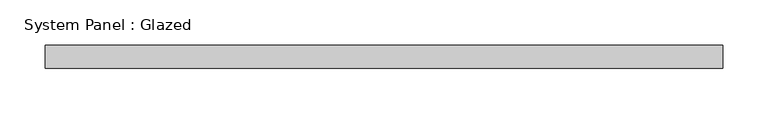
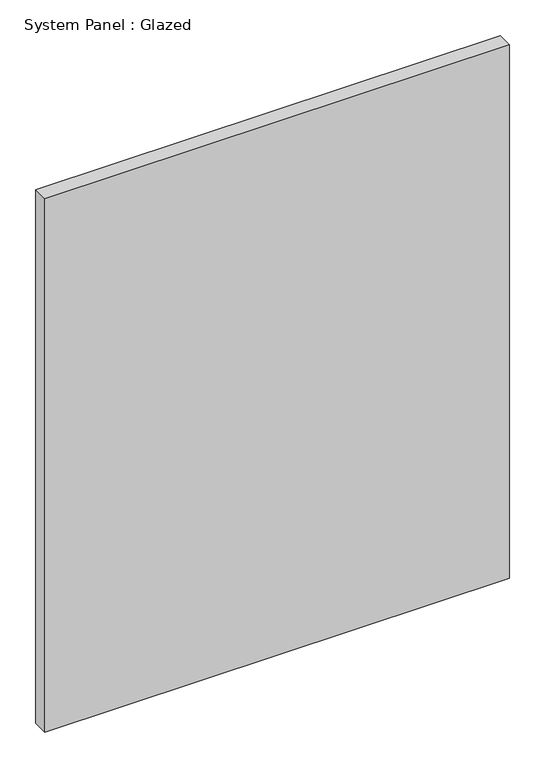
"""IFC4 building model written with IfcOpenShell, lengths in millimetres: plate geometry, System Panel : Glazed."""

from ifc_helpers import new_model, si_unit, origin, origin_with_axes, place, context, project, spatial, polyline, outline, extrude, source, transform, mapped, element, save


def system_panel_glazed_12683933(model_context):
    return source(origin(), model_context, "Body", "SweptSolid", [
        extrude(outline(polyline([(374.65, 19.05), (-374.65, 19.05), (-374.65, 44.45), (374.65, 44.45), (374.65, 19.05)])), origin_with_axes(), (0.0, 0.0, 1.0), 909.366916),
    ])


if __name__ == "__main__":
    model = new_model("IFC4")
    model_context = context("Model", 3, world=origin())
    ifc_project = project(units=[si_unit("LENGTHUNIT", "METRE", prefix="MILLI")], contexts=[model_context])
    site = spatial("IfcSite", under=ifc_project)
    building = spatial("IfcBuilding", under=site)
    placement = place(None, origin())
    system_panel_glazed_shape = system_panel_glazed_12683933(model_context)
    element("IfcPlate", 1, ObjectType="System Panel : Glazed", at=placement, inside=building, context=model_context, shape_type="MappedRepresentation", body=[
        mapped(system_panel_glazed_shape, transform((0.0, 0.0, 0.0), x_axis=(1.0, 0.0, 0.0), y_axis=(0.0, 1.0, 0.0), z_axis=(0.0, 0.0, 1.0))),
    ])
    save(model, "model.ifc")

# Revit data of these elements
# Type "System Panel : Glazed"
#   Construction Type Id = "GSP4R"
#   Analytic Construction = "1/8 in Pilkington single glazing"
#   Visual Light Transmittance = 0.9
#   Solar Heat Gain Coefficient = 0.86
#   Heat Transfer Coefficient (U) = 1.18115 BTU/(h·ft²·°F)
#   Define Thermal Properties by = 1
# Element 1 (IfcPlate, "System Panel : Glazed")
#   Materials on its faces: "Glass"
# Materials
#   "Glass": class "Glass", colour RGB 0 128 192, transparency 0.75, Description = "Soda Lime Glass", Cost = 0
